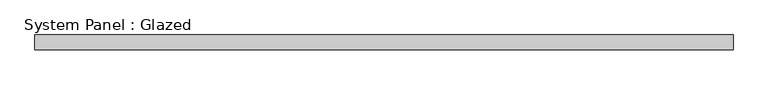
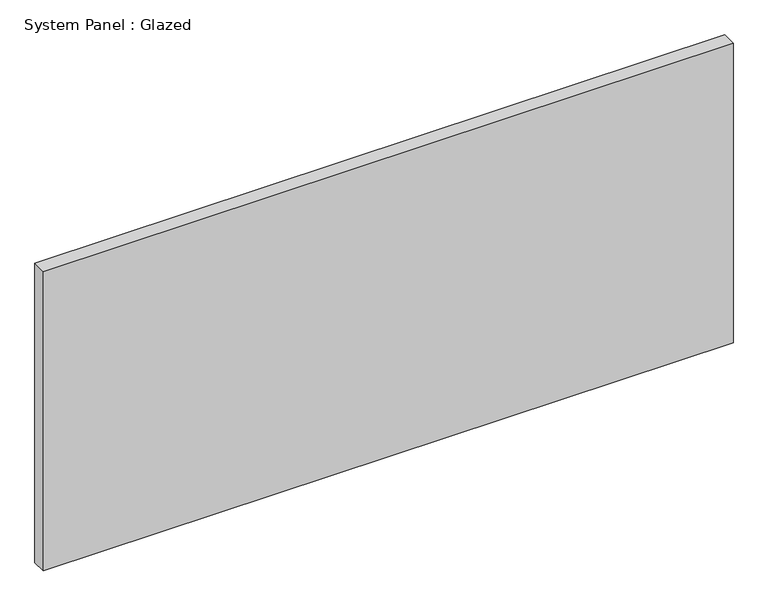
"""IFC4 building model written with IfcOpenShell, lengths in millimetres: plate geometry, System Panel : Glazed."""

from ifc_helpers import new_model, si_unit, origin, origin_with_axes, place, context, project, spatial, polyline, outline, extrude, source, transform, mapped, element, save


def system_panel_glazed_5475d124(model_context):
    return source(origin(), model_context, "Body", "SweptSolid", [
        extrude(outline(polyline([(595.3125, 19.05), (-595.3125, 19.05), (-595.3125, 44.45), (595.3125, 44.45), (595.3125, 19.05)])), origin_with_axes(), (0.0, 0.0, 1.0), 546.1),
    ])


if __name__ == "__main__":
    model = new_model("IFC4")
    model_context = context("Model", 3, world=origin())
    ifc_project = project(units=[si_unit("LENGTHUNIT", "METRE", prefix="MILLI")], contexts=[model_context])
    site = spatial("IfcSite", under=ifc_project)
    building = spatial("IfcBuilding", under=site)
    placement = place(None, origin())
    system_panel_glazed_shape = system_panel_glazed_5475d124(model_context)
    element("IfcPlate", 1, ObjectType="System Panel : Glazed", at=placement, inside=building, context=model_context, shape_type="MappedRepresentation", body=[
        mapped(system_panel_glazed_shape, transform((0.0, 0.0, 0.0), x_axis=(1.0, 0.0, 0.0), y_axis=(0.0, 1.0, 0.0), z_axis=(0.0, 0.0, 1.0))),
    ])
    save(model, "model.ifc")

# Revit data of these elements
# Type "System Panel : Glazed"
#   Construction Type Id = "GSP4R"
#   Analytic Construction = "1/8 in Pilkington single glazing"
#   Visual Light Transmittance = 0.9
#   Solar Heat Gain Coefficient = 0.86
#   Heat Transfer Coefficient (U) = 1.18115 BTU/(h·ft²·°F)
# Element 1 (IfcPlate, "System Panel : Glazed")
#   Materials on its faces: "Glass"
# Materials
#   "Glass": class "Glass", colour RGB 0 128 192, transparency 0.75, Description = "Soda Lime Glass", Cost = 0
